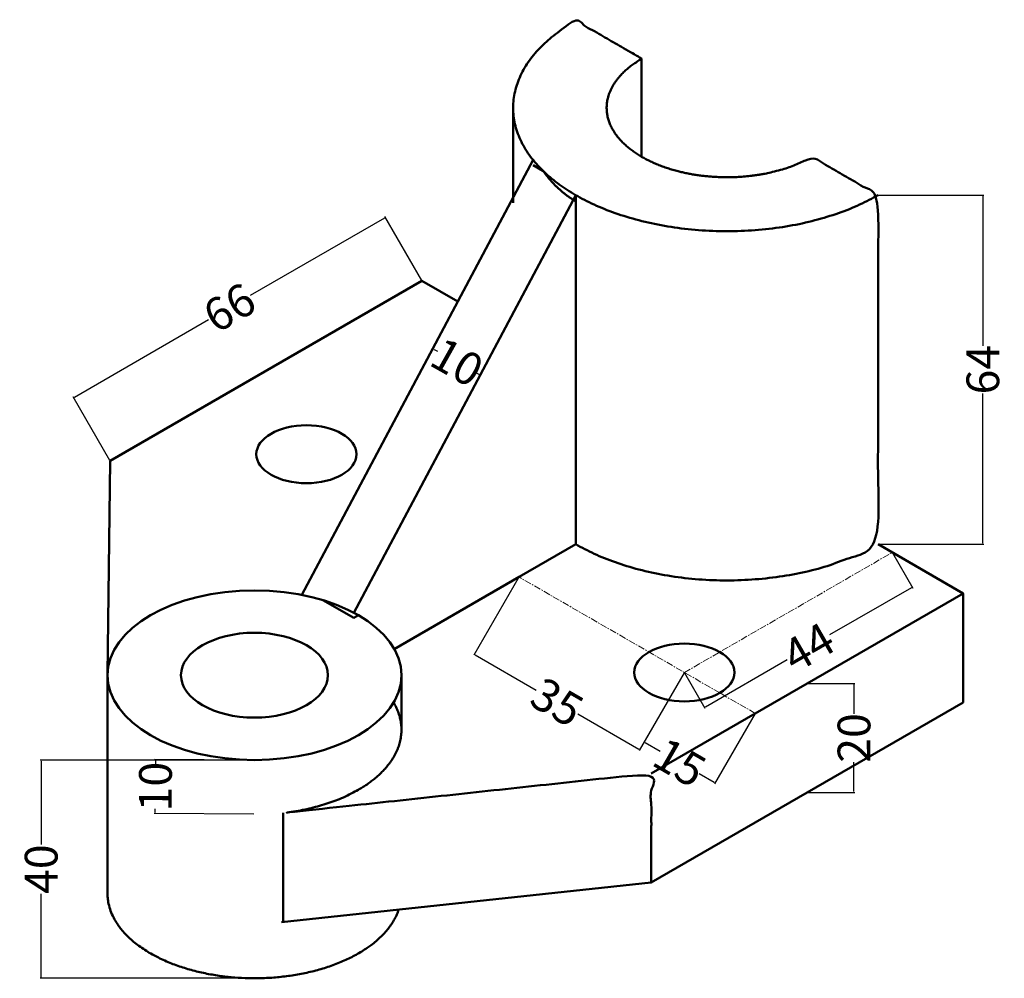
# Model space of a CAD drawing. Units: millimetres. Extents: x 35 to 215, y -3 to 172.
import ezdxf

# ---------------------------------------------------------------- set-up
doc = ezdxf.new("R2010")
doc.units = ezdxf.units.MM
doc.header["$MEASUREMENT"] = 0
doc.linetypes.add('CENTER', pattern=[2, 1.25, -0.25, 0.25, -0.25])
for name, color, linetype, lineweight in [('M-CNTR', 1, 'CENTER', 18), ('M-DIMS', 2, 'Continuous', 25), ('M-OUTL', 7, 'Continuous', 50)]:
    doc.layers.add(name, color=color, linetype=linetype, lineweight=lineweight)
doc.styles.get("Standard").update_dxf_attribs({"font": 'arial.ttf'})
doc.dimstyles.get("Standard").update_dxf_attribs({"dimtxt": 6, "dimasz": 0.18, "dimexe": 0.18, "dimexo": 0.0625, "dimgap": 0.09, "dimtad": 0, "dimtoh": 1, "dimdec": 0, "dimzin": 0, "dimdsep": 46, "dimtxsty": 'Standard', "dimcen": 0.09, "dimadec": 0, "dimazin": 0, "dimtfac": 1, "dimtdec": 0, "dimtofl": 0, "dimtmove": 0, "dimatfit": 3, "dimfxl": 1, "dimtolj": 1, "dimtzin": 0, "dimarcsym": 0})

# ---------------------------------------------------------------- blocks, each defined once
blk = doc.blocks.new('*D1')
at = {"layer": 'Defpoints', "color": 0, "transparency": 16777216}
for p in [(77.59, 36.62), (38.49, -3.38), (77.59, -3.38)]:
    blk.add_point(p, dxfattribs=at)
at = {"layer": 'M-DIMS', "color": 0, "lineweight": -2, "transparency": 16777216}
for p, q in [((77.53, 36.62), (38.31, 36.62)), ((38.49, 36.44), (38.49, 21.12)), ((38.49, -3.2), (38.49, 12.12)), ((77.53, -3.38), (38.31, -3.38))]:
    blk.add_line(p, q, dxfattribs=at)
at = {"layer": 'M-DIMS', "color": 0, "transparency": 16777216}
for points in [[(38.46, 36.44), (38.52, 36.44), (38.49, 36.62)], [(38.46, -3.2), (38.52, -3.2), (38.49, -3.38)]]:
    blk.add_solid(points, dxfattribs=at)
at = {"layer": 'M-DIMS', "color": 0, "transparency": 16777216, "insert": (38.49, 16.62), "char_height": 6, "attachment_point": 5, "rotation": 90}
blk.add_mtext('\\A1;40', dxfattribs=at)
blk = doc.blocks.new('*D2')
at = {"layer": 'Defpoints', "color": 0, "transparency": 16777216}
for p in [(77.59, 36.62), (59.4, 26.8), (77.54, 26.7)]:
    blk.add_point(p, dxfattribs=at)
at = {"layer": 'M-DIMS', "color": 0, "lineweight": -2, "transparency": 16777216}
for p, q in [((77.53, 36.62), (59.27, 36.71)), ((59.45, 36.53), (59.45, 35.85)), ((59.4, 26.98), (59.4, 27.66)), ((77.48, 26.7), (59.22, 26.8))]:
    blk.add_line(p, q, dxfattribs=at)
at = {"layer": 'M-DIMS', "color": 0, "transparency": 16777216}
for points in [[(59.42, 36.53), (59.48, 36.53), (59.45, 36.71)], [(59.37, 26.98), (59.43, 26.98), (59.4, 26.8)]]:
    blk.add_solid(points, dxfattribs=at)
at = {"layer": 'M-DIMS', "color": 0, "transparency": 16777216, "insert": (59.43, 31.75), "char_height": 6, "attachment_point": 5, "rotation": 89.6962}
blk.add_mtext('\\A1;10', dxfattribs=at)
blk = doc.blocks.new('*D3')
at = {"layer": 'Defpoints', "color": 0, "transparency": 16777216}
for p in [(107.47, 106.77), (119.08, 107.11), (116.16, 101.9)]:
    blk.add_point(p, dxfattribs=at)
at = {"layer": 'M-DIMS', "color": 0, "lineweight": -2, "transparency": 16777216}
for p, q in [((107.5, 106.83), (110.49, 112.14)), ((110.55, 111.9), (111.17, 111.55)), ((116.19, 101.95), (119.17, 107.27)), ((118.93, 107.2), (118.31, 107.55))]:
    blk.add_line(p, q, dxfattribs=at)
at = {"layer": 'M-DIMS', "color": 0, "transparency": 16777216}
for points in [[(110.57, 111.93), (110.54, 111.87), (110.4, 111.99)], [(118.94, 107.23), (118.91, 107.18), (119.08, 107.11)]]:
    blk.add_solid(points, dxfattribs=at)
at = {"layer": 'M-DIMS', "color": 0, "transparency": 16777216, "insert": (114.74, 109.55), "char_height": 6, "attachment_point": 5, "rotation": 330.7073}
blk.add_mtext('\\A1;10', dxfattribs=at)
blk = doc.blocks.new('*D4')
at = {"layer": 'Defpoints', "color": 0, "transparency": 16777216}
for p in [(178.92, 50.67), (178.92, 30.67), (187.49, 30.67)]:
    blk.add_point(p, dxfattribs=at)
at = {"layer": 'M-DIMS', "color": 0, "lineweight": -2, "transparency": 16777216}
for p, q in [((178.98, 50.67), (187.67, 50.67)), ((187.49, 50.49), (187.49, 45.1)), ((187.49, 30.85), (187.49, 36.25)), ((178.98, 30.67), (187.67, 30.67))]:
    blk.add_line(p, q, dxfattribs=at)
at = {"layer": 'M-DIMS', "color": 0, "transparency": 16777216}
for points in [[(187.46, 50.49), (187.52, 50.49), (187.49, 50.67)], [(187.46, 30.85), (187.52, 30.85), (187.49, 30.67)]]:
    blk.add_solid(points, dxfattribs=at)
at = {"layer": 'M-DIMS', "color": 0, "transparency": 16777216, "insert": (187.49, 40.67), "char_height": 6, "attachment_point": 5, "rotation": 90}
blk.add_mtext('\\A1;20', dxfattribs=at)
blk = doc.blocks.new('*D5')
at = {"layer": 'Defpoints', "color": 0, "transparency": 16777216}
for p in [(126.09, 70.17), (117.9, 55.99), (156.4, 52.67)]:
    blk.add_point(p, dxfattribs=at)
at = {"layer": 'M-DIMS', "color": 0, "lineweight": -2, "transparency": 16777216}
for p, q in [((126.06, 70.12), (117.81, 55.84)), ((118.06, 55.9), (129.24, 49.45)), ((156.37, 52.62), (148.13, 38.34)), ((148.06, 38.58), (136.88, 45.04))]:
    blk.add_line(p, q, dxfattribs=at)
at = {"layer": 'M-DIMS', "color": 0, "transparency": 16777216}
for points in [[(118.08, 55.93), (118.05, 55.88), (117.9, 55.99)], [(148.07, 38.61), (148.04, 38.56), (148.22, 38.49)]]:
    blk.add_solid(points, dxfattribs=at)
at = {"layer": 'M-DIMS', "color": 0, "transparency": 16777216, "insert": (133.06, 47.24), "char_height": 6, "attachment_point": 5, "rotation": 330}
blk.add_mtext('\\A1;35', dxfattribs=at)
blk = doc.blocks.new('*D6')
at = {"layer": 'Defpoints', "color": 0, "transparency": 16777216}
for p in [(194.51, 74.67), (198.19, 68.29), (156.4, 52.67)]:
    blk.add_point(p, dxfattribs=at)
at = {"layer": 'M-DIMS', "color": 0, "lineweight": -2, "transparency": 16777216}
for p, q in [((194.54, 74.62), (198.28, 68.14)), ((198.03, 68.2), (183.03, 59.54)), ((160.24, 46.38), (175.24, 55.05)), ((156.43, 52.62), (160.17, 46.14))]:
    blk.add_line(p, q, dxfattribs=at)
at = {"layer": 'M-DIMS', "color": 0, "transparency": 16777216}
for points in [[(198.02, 68.23), (198.05, 68.18), (198.19, 68.29)], [(160.23, 46.41), (160.26, 46.36), (160.08, 46.29)]]:
    blk.add_solid(points, dxfattribs=at)
at = {"layer": 'M-DIMS', "color": 0, "transparency": 16777216, "insert": (179.14, 57.29), "char_height": 6, "attachment_point": 5, "rotation": 30}
blk.add_mtext('\\A1;44', dxfattribs=at)
blk = doc.blocks.new('*D7')
at = {"layer": 'Defpoints', "color": 0, "transparency": 16777216}
for p in [(156.4, 52.67), (169.39, 45.17), (162.03, 32.42)]:
    blk.add_point(p, dxfattribs=at)
at = {"layer": 'M-DIMS', "color": 0, "lineweight": -2, "transparency": 16777216}
for p, q in [((156.37, 52.62), (148.95, 39.76)), ((169.36, 45.12), (161.94, 32.26)), ((149.19, 39.83), (151.96, 38.23)), ((161.87, 32.51), (159.11, 34.1))]:
    blk.add_line(p, q, dxfattribs=at)
at = {"layer": 'M-DIMS', "color": 0, "transparency": 16777216}
for points in [[(149.21, 39.85), (149.18, 39.8), (149.04, 39.92)], [(161.89, 32.53), (161.86, 32.48), (162.03, 32.42)]]:
    blk.add_solid(points, dxfattribs=at)
at = {"layer": 'M-DIMS', "color": 0, "transparency": 16777216, "insert": (155.53, 36.17), "char_height": 6, "attachment_point": 5, "rotation": 330}
blk.add_mtext('\\A1;15', dxfattribs=at)
blk = doc.blocks.new('*D8')
at = {"layer": 'Defpoints', "color": 0, "transparency": 16777216}
for p in [(101.58, 136.06), (108.28, 124.46), (51.12, 91.46)]:
    blk.add_point(p, dxfattribs=at)
at = {"layer": 'M-DIMS', "color": 0, "lineweight": -2, "transparency": 16777216}
for p, q in [((101.42, 135.97), (76.81, 121.76)), ((108.25, 124.51), (101.49, 136.22)), ((44.58, 103.15), (69.19, 117.36)), ((51.09, 91.51), (44.33, 103.22))]:
    blk.add_line(p, q, dxfattribs=at)
at = {"layer": 'M-DIMS', "color": 0, "transparency": 16777216}
for points in [[(101.41, 136), (101.44, 135.94), (101.58, 136.06)], [(44.56, 103.18), (44.59, 103.12), (44.42, 103.06)]]:
    blk.add_solid(points, dxfattribs=at)
at = {"layer": 'M-DIMS', "color": 0, "transparency": 16777216, "insert": (73, 119.56), "char_height": 6, "attachment_point": 5, "rotation": 30}
blk.add_mtext('\\A1;66', dxfattribs=at)
blk = doc.blocks.new('*D9')
at = {"layer": 'Defpoints', "color": 0, "transparency": 16777216}
for p in [(191.91, 140.17), (191.91, 76.17), (211.11, 76.17)]:
    blk.add_point(p, dxfattribs=at)
at = {"layer": 'M-DIMS', "color": 0, "lineweight": -2, "transparency": 16777216}
for p, q in [((191.97, 140.17), (211.29, 140.17)), ((211.11, 139.99), (211.11, 112.56)), ((211.11, 76.35), (211.11, 103.78)), ((191.97, 76.17), (211.29, 76.17))]:
    blk.add_line(p, q, dxfattribs=at)
at = {"layer": 'M-DIMS', "color": 0, "transparency": 16777216}
for points in [[(211.08, 139.99), (211.14, 139.99), (211.11, 140.17)], [(211.08, 76.35), (211.14, 76.35), (211.11, 76.17)]]:
    blk.add_solid(points, dxfattribs=at)
at = {"layer": 'M-DIMS', "color": 0, "transparency": 16777216, "insert": (211.11, 108.17), "char_height": 6, "attachment_point": 5, "rotation": 90}
blk.add_mtext('\\A1;64', dxfattribs=at)

msp = doc.modelspace()

# ---------------------------------------------------------------- linework, layer by layer
at = {"layer": 'M-CNTR'}
msp.add_line((156.4, 52.67), (194.51, 74.67), dxfattribs=at)
msp.add_lwpolyline([(169.39, 45.17), (162.9, 48.92), (126.09, 70.17)], dxfattribs=at)
at = {"layer": 'M-OUTL'}
for p, q in [((148.56, 165.15), (148.56, 147.2)), ((146.31, 163.61), (146.31, 163.61)), ((125, 156.17), (125, 138.76)), ((128.65, 146.65), (86.3, 66.9)), ((130.48, 144.64), (128.69, 145.67)), ((136.48, 140.17), (95.83, 63.62)), ((136.48, 76.17), (136.48, 140.17)), ((108.28, 124.46), (51.12, 91.46)), ((114.85, 120.66), (108.28, 124.46)), ((51.12, 91.46), (50.65, 52.28)), ((191.91, 76.17), (207.5, 67.17)), ((90.1, 65.95), (95.78, 62.67)), ((95.78, 62.67), (96.65, 63.17)), ((104.54, 42.17), (104.54, 52.17)), ((82.88, 6.92), (82.88, 26.92))]:
    msp.add_line(p, q, dxfattribs=at)
for points in [[(130.48, 144.64), (130.53, 144.57), (130.58, 144.5), (130.63, 144.42), (130.69, 144.35), (130.74, 144.28), (130.79, 144.2), (130.85, 144.13), (130.9, 144.06), (130.95, 143.99), (131.01, 143.92), (131.06, 143.85), (131.12, 143.78), (131.17, 143.71), (131.23, 143.64), (131.28, 143.57), (131.34, 143.5), (131.4, 143.43), (131.45, 143.36), (131.51, 143.29), (131.56, 143.22), (131.62, 143.16), (131.68, 143.09), (131.74, 143.02), (131.79, 142.96), (131.85, 142.89), (131.91, 142.82), (131.97, 142.76), (132.02, 142.69), (132.08, 142.63), (132.14, 142.56), (132.2, 142.5), (132.26, 142.44), (132.32, 142.37), (132.38, 142.31), (132.44, 142.24), (132.5, 142.18), (132.56, 142.12), (132.62, 142.06), (132.68, 142), (132.74, 141.94), (132.8, 141.87), (132.86, 141.81), (132.93, 141.75), (132.99, 141.69), (133.05, 141.64), (133.11, 141.58), (133.17, 141.52), (133.24, 141.46), (133.3, 141.4), (133.36, 141.34), (133.43, 141.28), (133.49, 141.23), (133.55, 141.17), (133.62, 141.11), (133.68, 141.06), (133.75, 141), (133.81, 140.95), (133.88, 140.89), (133.94, 140.84), (134.01, 140.78), (134.07, 140.73), (134.14, 140.67), (134.2, 140.62), (134.27, 140.57), (134.33, 140.51), (134.4, 140.46), (134.47, 140.41), (134.53, 140.36), (134.6, 140.31), (134.67, 140.25), (134.74, 140.2), (134.8, 140.15), (134.87, 140.1), (134.94, 140.05), (135.01, 140), (135.07, 139.96), (135.14, 139.91), (135.21, 139.86), (135.28, 139.81), (135.35, 139.76), (135.42, 139.72), (135.49, 139.67), (135.56, 139.62), (135.63, 139.58), (135.7, 139.53), (135.77, 139.49), (135.84, 139.44), (135.91, 139.4), (135.98, 139.35), (136.05, 139.31), (136.12, 139.26), (136.2, 139.22), (136.27, 139.18), (136.34, 139.13), (136.41, 139.09), (136.48, 139.05)], [(136.48, 76.17), (126.09, 70.17), (103.22, 56.97)], [(150.34, 34.17), (207.5, 67.17), (207.5, 47.17), (150.34, 14.17), (82.53, 6.88)]]:
    msp.add_lwpolyline(points, dxfattribs=at)
for centre, major_axis in [((87.12, 92.67), (-9.19, 0)), ((77.59, 52.17), (-26.94, 0)), ((77.59, 52.17), (-13.47, 0)), ((156.4, 52.67), (-9.19, 0))]:
    msp.add_ellipse(centre, major_axis=major_axis, ratio=0.57735, dxfattribs=at)
for centre, start_param, end_param in [((77.59, 12.17), 10.719311, 10.727325), ((76.03, 12.2), 4.408628, 4.411985)]:
    msp.add_ellipse(centre, major_axis=(-26.94, 0), ratio=0.57735, start_param=start_param, end_param=end_param, dxfattribs=at)
for points, weights, knots in [([(191.91, 140.17), (164.2, 124.17), (136.48, 140.17), (108.77, 156.17), (136.48, 172.17), (142.55, 168.67), (148.61, 165.17), (139.61, 159.98), (142.9, 152.88), (146.2, 145.78), (158.49, 143.88), (170.78, 141.98), (179.78, 147.17), (185.85, 143.67), (191.91, 140.17), (191.91, 108.17), (191.91, 76.17), (164.2, 60.17), (136.48, 76.17)], [1, 0.707106781187, 1, 0.707106781187, 1, 1, 1, 0.866025403784, 1, 0.866025403784, 1, 0.866025403784, 1, 1, 1, 1, 1, 0.707106781187, 1], [0, 0, 0, 1.570796, 1.570796, 3.141593, 3.141593, 4.141593, 4.141593, 5.18879, 5.18879, 6.235988, 6.235988, 7.283185, 7.283185, 8.283185, 8.283185, 9.283185, 9.283185, 10.853982, 10.853982, 10.853982]), ([(50.65, 52.17), (50.65, 32.17), (50.65, 12.17), (50.65, -1.95), (75, -3.31), (99.35, -4.67), (104.04, 9.19)], [1, 1, 1, 0.740343816394, 1, 0.740343816394, 1], [0, 0, 0, 1, 1, 2.474429, 2.474429, 3.948859, 3.948859, 3.948859]), ([(150.34, 14.17), (150.34, 24.17), (150.34, 34.17), (116.43, 30.53), (82.53, 26.88), (94.63, 28.18), (100.85, 34.31), (107.06, 40.44), (103.11, 47.17)], [1, 1, 1, 1, 1, 0.909606353896, 1, 0.909606353896, 1], [0, 0, 0, 1, 1, 2, 2, 2.856921, 2.856921, 3.713843, 3.713843, 3.713843])]:
    msp.add_rational_spline(points, weights, degree=2, knots=knots, dxfattribs=at)

# ---------------------------------------------------------------- dimensions: what is measured, and where the dimension line sits
at = {"layer": 'M-DIMS'}
for p1, p2, distance, picture, middle in [((191.91, 140.17), (191.91, 76.17), 19.2, '*D9', (211.11, 108.17)), ((51.12, 91.46), (108.28, 124.46), 13.4, '*D8', (73, 119.56)), ((107.47, 106.77), (116.16, 101.9), 5.98, '*D3', (114.74, 109.55)), ((156.4, 52.67), (194.51, 74.67), -7.37, '*D6', (179.14, 57.29)), ((156.4, 52.67), (126.09, 70.17), 16.37, '*D5', (133.06, 47.24)), ((156.4, 52.67), (169.39, 45.17), -14.73, '*D7', (155.53, 36.17)), ((178.92, 50.67), (178.92, 30.67), 8.57, '*D4', (187.49, 40.67)), ((77.59, 36.62), (77.59, -3.38), -39.1, '*D1', (38.49, 16.62)), ((77.59, 36.62), (77.54, 26.7), -18.14, '*D2', (59.43, 31.75))]:
    dim = msp.add_aligned_dim(p1=p1, p2=p2, distance=distance, dimstyle='Standard', override={"dimclrd": 0, "dimclre": 0, "dimclrt": 0}, dxfattribs=at)
    dim.commit()
    dim.dimension.update_dxf_attribs({"geometry": picture, "text_midpoint": middle})

doc.saveas('drawing.dxf')
